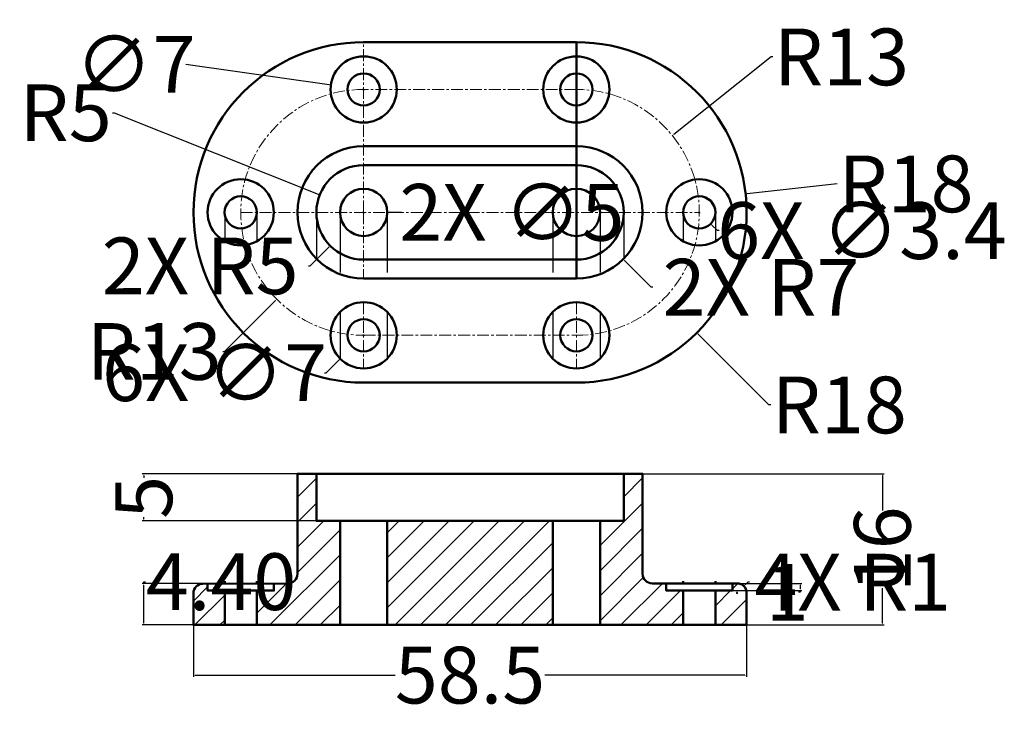
# Model space of a CAD drawing. Units: millimetres. Extents: x 26 to 130, y 11 to 85.
import ezdxf

# ---------------------------------------------------------------- set-up
doc = ezdxf.new("R2010")
doc.units = ezdxf.units.MM
doc.header["$MEASUREMENT"] = 0
doc.linetypes.add('CENTER', pattern=[2, 1.25, -0.25, 0.25, -0.25])
doc.linetypes.add('HIDDEN', pattern=[9.525, 6.35, -3.175])
for name, color, linetype, lineweight in [('M-CNTR', 1, 'CENTER', 18), ('M-DIMS', 2, 'Continuous', 25), ('M-HATC', 8, 'Continuous', 18), ('M-HIDN', 4, 'HIDDEN', 25), ('M-OUTL', 7, 'Continuous', 50)]:
    doc.layers.add(name, color=color, linetype=linetype, lineweight=lineweight)
doc.styles.get("Standard").update_dxf_attribs({"font": 'arial.ttf'})
doc.dimstyles.get("Standard").update_dxf_attribs({"dimtxt": 6, "dimasz": 0.18, "dimexe": 0.18, "dimexo": 0.0625, "dimgap": 0.09, "dimtad": 0, "dimtoh": 1, "dimdec": 0, "dimzin": 0, "dimdsep": 46, "dimtxsty": 'Standard', "dimcen": 0.09, "dimadec": 0, "dimazin": 0, "dimtfac": 1, "dimtdec": 0, "dimtofl": 0, "dimtmove": 0, "dimatfit": 3, "dimfxl": 1, "dimtolj": 1, "dimtzin": 0, "dimarcsym": 0})

# ---------------------------------------------------------------- blocks, each defined once
blk = doc.blocks.new('*D1')
at = {"layer": 'Defpoints', "color": 0, "transparency": 16777216}
for p in [(94.96, 72.32), (84.8, 64.21)]:
    blk.add_point(p, dxfattribs=at)
at = {"layer": 'M-DIMS', "color": 0, "lineweight": -2, "transparency": 16777216}
for p, q in [((105.4, 80.65), (95.1, 72.43)), ((105.58, 80.65), (105.4, 80.65)), ((84.71, 64.21), (84.89, 64.21)), ((84.8, 64.12), (84.8, 64.3))]:
    blk.add_line(p, q, dxfattribs=at)
at = {"layer": 'M-DIMS', "color": 0, "transparency": 16777216}
blk.add_solid([(95.08, 72.45), (95.12, 72.4), (94.96, 72.32)], dxfattribs=at)
at = {"layer": 'M-DIMS', "color": 0, "transparency": 16777216, "insert": (112.84, 80.65), "char_height": 6, "attachment_point": 5}
blk.add_mtext('\\A1;R13', dxfattribs=at)
blk = doc.blocks.new('*D2')
at = {"layer": 'Defpoints', "color": 0, "transparency": 16777216}
for p in [(102.69, 66.16), (84.8, 64.21)]:
    blk.add_point(p, dxfattribs=at)
at = {"layer": 'M-DIMS', "color": 0, "lineweight": -2, "transparency": 16777216}
for p, q in [((112.39, 67.22), (102.87, 66.18)), ((84.71, 64.21), (84.89, 64.21)), ((84.8, 64.12), (84.8, 64.3))]:
    blk.add_line(p, q, dxfattribs=at)
at = {"layer": 'M-DIMS', "color": 0, "transparency": 16777216}
blk.add_solid([(102.87, 66.21), (102.88, 66.15), (102.69, 66.16)], dxfattribs=at)
at = {"layer": 'M-DIMS', "color": 0, "transparency": 16777216, "insert": (119.66, 67.22), "char_height": 6, "attachment_point": 5}
blk.add_mtext('\\A1;R18', dxfattribs=at)
blk = doc.blocks.new('*D3')
at = {"layer": 'Defpoints', "color": 0, "transparency": 16777216}
for p in [(57.66, 66.06), (62.3, 64.21)]:
    blk.add_point(p, dxfattribs=at)
at = {"layer": 'M-DIMS', "color": 0, "lineweight": -2, "transparency": 16777216}
for p, q in [((35.74, 74.74), (35.92, 74.74)), ((35.92, 74.74), (57.49, 66.13)), ((62.21, 64.21), (62.39, 64.21)), ((62.3, 64.12), (62.3, 64.3))]:
    blk.add_line(p, q, dxfattribs=at)
at = {"layer": 'M-DIMS', "color": 0, "transparency": 16777216}
blk.add_solid([(57.5, 66.16), (57.48, 66.1), (57.66, 66.06)], dxfattribs=at)
at = {"layer": 'M-DIMS', "color": 0, "transparency": 16777216, "insert": (30.79, 74.74), "char_height": 6, "attachment_point": 5}
blk.add_mtext('\\A1;R5', dxfattribs=at)
blk = doc.blocks.new('*D4')
at = {"layer": 'Defpoints', "color": 0, "transparency": 16777216}
for p in [(89.8, 36.57), (89.8, 20.57), (117.16, 20.57)]:
    blk.add_point(p, dxfattribs=at)
at = {"layer": 'M-DIMS', "color": 0, "lineweight": -2, "transparency": 16777216}
for p, q in [((89.86, 36.57), (117.34, 36.57)), ((117.16, 36.39), (117.16, 32.68)), ((117.16, 20.75), (117.16, 24.47)), ((89.86, 20.57), (117.34, 20.57))]:
    blk.add_line(p, q, dxfattribs=at)
at = {"layer": 'M-DIMS', "color": 0, "transparency": 16777216}
for points in [[(117.13, 36.39), (117.19, 36.39), (117.16, 36.57)], [(117.13, 20.75), (117.19, 20.75), (117.16, 20.57)]]:
    blk.add_solid(points, dxfattribs=at)
at = {"layer": 'M-DIMS', "color": 0, "transparency": 16777216, "insert": (117.16, 28.57), "char_height": 6, "attachment_point": 5, "rotation": 90}
blk.add_mtext('\\A1;16', dxfattribs=at)
blk = doc.blocks.new('*D5')
at = {"layer": 'Defpoints', "color": 0, "transparency": 16777216}
for p in [(97.3, 24.97), (97.3, 24.21), (108.48, 24.21)]:
    blk.add_point(p, dxfattribs=at)
at = {"layer": 'M-DIMS', "color": 0, "lineweight": -2, "transparency": 16777216}
for p, q in [((97.36, 24.97), (108.66, 24.97)), ((97.36, 24.21), (108.66, 24.21)), ((108.48, 24.03), (108.3, 24.03)), ((108.48, 24.79), (108.48, 24.39)), ((108.48, 24.21), (108.48, 24.03))]:
    blk.add_line(p, q, dxfattribs=at)
at = {"layer": 'M-DIMS', "color": 0, "transparency": 16777216}
for points in [[(108.45, 24.79), (108.51, 24.79), (108.48, 24.97)], [(108.45, 24.39), (108.51, 24.39), (108.48, 24.21)]]:
    blk.add_solid(points, dxfattribs=at)
at = {"layer": 'M-DIMS', "color": 0, "transparency": 16777216, "insert": (107.11, 24.03), "char_height": 6, "attachment_point": 5}
blk.add_mtext('\\A1;1', dxfattribs=at)
blk = doc.blocks.new('*D6')
at = {"layer": 'Defpoints', "color": 0, "transparency": 16777216}
for p in [(58.84, 77.7), (65.77, 76.72)]:
    blk.add_point(p, dxfattribs=at)
at = {"layer": 'M-DIMS', "color": 0, "lineweight": -2, "transparency": 16777216}
for p, q in [((43.48, 79.87), (58.66, 77.72)), ((62.21, 77.21), (62.39, 77.21)), ((62.3, 77.12), (62.3, 77.3))]:
    blk.add_line(p, q, dxfattribs=at)
at = {"layer": 'M-DIMS', "color": 0, "transparency": 16777216}
blk.add_solid([(58.66, 77.75), (58.65, 77.69), (58.84, 77.7)], dxfattribs=at)
at = {"layer": 'M-DIMS', "color": 0, "transparency": 16777216, "insert": (38.16, 79.87), "char_height": 6, "attachment_point": 5}
blk.add_mtext('\\A1;∅7', dxfattribs=at)
blk = doc.blocks.new('HOLE-CBORE-3.4X7')
for radius in [3.5, 1.7]:
    blk.add_circle((62.3, 77.21), radius)
blk = doc.blocks.new('*D8')
at = {"layer": 'Defpoints', "color": 0, "transparency": 16777216}
for p in [(44.3, 20.57), (102.8, 20.57), (102.8, 15.27)]:
    blk.add_point(p, dxfattribs=at)
at = {"layer": 'M-DIMS', "color": 0, "lineweight": -2, "transparency": 16777216}
for p, q in [((44.3, 20.51), (44.3, 15.09)), ((102.8, 20.51), (102.8, 15.09)), ((44.48, 15.27), (65.65, 15.27)), ((102.62, 15.27), (81.46, 15.27))]:
    blk.add_line(p, q, dxfattribs=at)
at = {"layer": 'M-DIMS', "color": 0, "transparency": 16777216}
for points in [[(44.48, 15.3), (44.48, 15.24), (44.3, 15.27)], [(102.62, 15.3), (102.62, 15.24), (102.8, 15.27)]]:
    blk.add_solid(points, dxfattribs=at)
at = {"layer": 'M-DIMS', "color": 0, "transparency": 16777216, "insert": (73.55, 15.27), "char_height": 6, "attachment_point": 5}
blk.add_mtext('\\A1;58.5', dxfattribs=at)
blk = doc.blocks.new('*D9')
at = {"layer": 'Defpoints', "color": 0, "transparency": 16777216}
for p in [(39.05, 24.97), (54.31, 24.97), (44.3, 20.57)]:
    blk.add_point(p, dxfattribs=at)
at = {"layer": 'M-DIMS', "color": 0, "lineweight": -2, "transparency": 16777216}
for p, q in [((39.05, 24.97), (39.05, 25.15)), ((39.05, 25.15), (39.23, 25.15)), ((54.24, 24.97), (38.87, 24.97)), ((39.05, 20.75), (39.05, 24.79)), ((44.24, 20.57), (38.87, 20.57))]:
    blk.add_line(p, q, dxfattribs=at)
at = {"layer": 'M-DIMS', "color": 0, "transparency": 16777216}
for points in [[(39.02, 24.79), (39.08, 24.79), (39.05, 24.97)], [(39.02, 20.75), (39.08, 20.75), (39.05, 20.57)]]:
    blk.add_solid(points, dxfattribs=at)
at = {"layer": 'M-DIMS', "color": 0, "transparency": 16777216, "insert": (47.22, 25.15), "char_height": 6, "attachment_point": 5}
blk.add_mtext('\\A1;4.40', dxfattribs=at)
blk = doc.blocks.new('*D10')
at = {"layer": 'Defpoints', "color": 0, "transparency": 16777216}
for p in [(57.3, 36.57), (39.05, 31.57), (57.3, 31.57)]:
    blk.add_point(p, dxfattribs=at)
at = {"layer": 'M-DIMS', "color": 0, "lineweight": -2, "transparency": 16777216}
for p, q in [((57.24, 36.57), (38.87, 36.57)), ((39.05, 36.39), (39.05, 36.15)), ((57.24, 31.57), (38.87, 31.57)), ((39.05, 31.75), (39.05, 31.99))]:
    blk.add_line(p, q, dxfattribs=at)
at = {"layer": 'M-DIMS', "color": 0, "transparency": 16777216}
for points in [[(39.02, 36.39), (39.08, 36.39), (39.05, 36.57)], [(39.02, 31.75), (39.08, 31.75), (39.05, 31.57)]]:
    blk.add_solid(points, dxfattribs=at)
at = {"layer": 'M-DIMS', "color": 0, "transparency": 16777216, "insert": (39.05, 34.07), "char_height": 6, "attachment_point": 5, "rotation": 90}
blk.add_mtext('\\A1;5', dxfattribs=at)
blk = doc.blocks.new('*D11')
at = {"layer": 'Defpoints', "color": 0, "transparency": 16777216}
for p in [(84.8, 64.21), (97.53, 51.48)]:
    blk.add_point(p, dxfattribs=at)
at = {"layer": 'M-DIMS', "color": 0, "lineweight": -2, "transparency": 16777216}
for p, q in [((84.71, 64.21), (84.89, 64.21)), ((84.8, 64.12), (84.8, 64.3)), ((105.17, 43.84), (97.66, 51.35)), ((105.35, 43.84), (105.17, 43.84))]:
    blk.add_line(p, q, dxfattribs=at)
at = {"layer": 'M-DIMS', "color": 0, "transparency": 16777216}
blk.add_solid([(97.68, 51.37), (97.64, 51.33), (97.53, 51.48)], dxfattribs=at)
at = {"layer": 'M-DIMS', "color": 0, "transparency": 16777216, "insert": (112.61, 43.84), "char_height": 6, "attachment_point": 5}
blk.add_mtext('\\A1;R18', dxfattribs=at)
blk = doc.blocks.new('*D12')
at = {"layer": 'Defpoints', "color": 0, "transparency": 16777216}
for p in [(62.3, 64.21), (53.11, 55.02)]:
    blk.add_point(p, dxfattribs=at)
at = {"layer": 'M-DIMS', "color": 0, "lineweight": -2, "transparency": 16777216}
for p, q in [((62.21, 64.21), (62.39, 64.21)), ((62.3, 64.12), (62.3, 64.3)), ((47.59, 49.5), (52.98, 54.89)), ((47.41, 49.5), (47.59, 49.5))]:
    blk.add_line(p, q, dxfattribs=at)
at = {"layer": 'M-DIMS', "color": 0, "transparency": 16777216}
blk.add_solid([(52.96, 54.91), (53, 54.87), (53.11, 55.02)], dxfattribs=at)
at = {"layer": 'M-DIMS', "color": 0, "transparency": 16777216, "insert": (40.15, 49.5), "char_height": 6, "attachment_point": 5}
blk.add_mtext('\\A1;R13', dxfattribs=at)
blk = doc.blocks.new('*D13')
at = {"layer": 'Defpoints', "color": 0, "transparency": 16777216}
for p in [(84.8, 64.21), (89.75, 59.26)]:
    blk.add_point(p, dxfattribs=at)
at = {"layer": 'M-DIMS', "color": 0, "lineweight": -2, "transparency": 16777216}
for p, q in [((84.71, 64.21), (84.89, 64.21)), ((84.8, 64.12), (84.8, 64.3)), ((92.72, 56.29), (89.88, 59.13)), ((92.9, 56.29), (92.72, 56.29))]:
    blk.add_line(p, q, dxfattribs=at)
at = {"layer": 'M-DIMS', "color": 0, "transparency": 16777216}
blk.add_solid([(89.9, 59.15), (89.86, 59.11), (89.75, 59.26)], dxfattribs=at)
at = {"layer": 'M-DIMS', "color": 0, "transparency": 16777216, "insert": (104.33, 56.29), "char_height": 6, "attachment_point": 5}
blk.add_mtext('\\A1;2X R7', dxfattribs=at)
blk = doc.blocks.new('*D14')
at = {"layer": 'Defpoints', "color": 0, "transparency": 16777216}
for p in [(62.3, 64.21), (58.76, 60.67)]:
    blk.add_point(p, dxfattribs=at)
at = {"layer": 'M-DIMS', "color": 0, "lineweight": -2, "transparency": 16777216}
for p, q in [((62.21, 64.21), (62.39, 64.21)), ((62.3, 64.12), (62.3, 64.3)), ((56.64, 58.55), (58.64, 60.55)), ((56.46, 58.55), (56.64, 58.55))]:
    blk.add_line(p, q, dxfattribs=at)
at = {"layer": 'M-DIMS', "color": 0, "transparency": 16777216}
blk.add_solid([(58.62, 60.57), (58.66, 60.53), (58.76, 60.67)], dxfattribs=at)
at = {"layer": 'M-DIMS', "color": 0, "transparency": 16777216, "insert": (45.01, 58.55), "char_height": 6, "attachment_point": 5}
blk.add_mtext('\\A1;2X R5', dxfattribs=at)
blk = doc.blocks.new('*D15')
at = {"layer": 'Defpoints', "color": 0, "transparency": 16777216}
for p in [(64.78, 53.68), (59.82, 48.73)]:
    blk.add_point(p, dxfattribs=at)
at = {"layer": 'M-DIMS', "color": 0, "lineweight": -2, "transparency": 16777216}
for p, q in [((62.21, 51.21), (62.39, 51.21)), ((62.3, 51.12), (62.3, 51.3)), ((58.34, 47.25), (59.7, 48.61)), ((58.16, 47.25), (58.34, 47.25))]:
    blk.add_line(p, q, dxfattribs=at)
at = {"layer": 'M-DIMS', "color": 0, "transparency": 16777216}
blk.add_solid([(59.68, 48.63), (59.72, 48.59), (59.82, 48.73)], dxfattribs=at)
at = {"layer": 'M-DIMS', "color": 0, "transparency": 16777216, "insert": (46.53, 47.25), "char_height": 6, "attachment_point": 5}
blk.add_mtext('\\A1;6X ∅7', dxfattribs=at)
blk = doc.blocks.new('*D16')
at = {"layer": 'Defpoints', "color": 0, "transparency": 16777216}
for p in [(96.6, 65.41), (99, 63)]:
    blk.add_point(p, dxfattribs=at)
at = {"layer": 'M-DIMS', "color": 0, "lineweight": -2, "transparency": 16777216}
for p, q in [((97.71, 64.21), (97.89, 64.21)), ((97.8, 64.12), (97.8, 64.3)), ((99.72, 62.28), (99.13, 62.87)), ((99.9, 62.28), (99.72, 62.28))]:
    blk.add_line(p, q, dxfattribs=at)
at = {"layer": 'M-DIMS', "color": 0, "transparency": 16777216}
blk.add_solid([(99.15, 62.89), (99.1, 62.85), (99, 63)], dxfattribs=at)
at = {"layer": 'M-DIMS', "color": 0, "transparency": 16777216, "insert": (115, 62.28), "char_height": 6, "attachment_point": 5}
blk.add_mtext('\\A1;6X ∅3.4', dxfattribs=at)
blk = doc.blocks.new('*D17')
at = {"layer": 'Defpoints', "color": 0, "transparency": 16777216}
for p in [(59.8, 64.21), (64.8, 64.21)]:
    blk.add_point(p, dxfattribs=at)
at = {"layer": 'M-DIMS', "color": 0, "lineweight": -2, "transparency": 16777216}
for p, q in [((62.21, 64.21), (62.39, 64.21)), ((62.3, 64.12), (62.3, 64.3)), ((66.3, 64.21), (64.98, 64.21))]:
    blk.add_line(p, q, dxfattribs=at)
at = {"layer": 'M-DIMS', "color": 0, "transparency": 16777216}
blk.add_solid([(64.98, 64.24), (64.98, 64.18), (64.8, 64.21)], dxfattribs=at)
at = {"layer": 'M-DIMS', "color": 0, "transparency": 16777216, "insert": (77.98, 64.21), "char_height": 6, "attachment_point": 5}
blk.add_mtext('\\A1;2X ∅5', dxfattribs=at)
blk = doc.blocks.new('*D18')
at = {"layer": 'Defpoints', "color": 0, "transparency": 16777216}
for p in [(101.8, 23.97), (102.51, 24.68)]:
    blk.add_point(p, dxfattribs=at)
at = {"layer": 'M-DIMS', "color": 0, "lineweight": -2, "transparency": 16777216}
for p, q in [((102.93, 25.1), (102.64, 24.81)), ((103.11, 25.1), (102.93, 25.1)), ((101.71, 23.97), (101.89, 23.97)), ((101.8, 23.88), (101.8, 24.06))]:
    blk.add_line(p, q, dxfattribs=at)
at = {"layer": 'M-DIMS', "color": 0, "transparency": 16777216}
blk.add_solid([(102.61, 24.83), (102.66, 24.79), (102.51, 24.68)], dxfattribs=at)
at = {"layer": 'M-DIMS', "color": 0, "transparency": 16777216, "insert": (114.03, 25.1), "char_height": 6, "attachment_point": 5}
blk.add_mtext('\\A1;4X R1', dxfattribs=at)

msp = doc.modelspace()

# ---------------------------------------------------------------- hatches: boundary and pattern name
at = {"layer": 'M-HATC'}
h = msp.add_hatch(dxfattribs=at)
h.set_pattern_fill('ANSI31', color=256, scale=15)
h.paths.add_polyline_path([(59.801, 31.572), (57.301, 31.572), (57.301, 36.572), (55.301, 36.572), (55.301, 25.968, -0.4128846), (54.306, 24.968), (52.801, 24.961), (52.801, 24.207), (51.001, 24.207), (51.001, 20.572), (59.801, 20.572)])
h.paths.add_polyline_path([(82.301, 31.572), (64.801, 31.572), (64.801, 20.572), (82.301, 20.572)])
h.paths.add_polyline_path([(94.301, 24.972), (92.801, 24.972, -0.4142136), (91.801, 25.972), (91.801, 36.572), (89.801, 36.572), (89.801, 31.572), (87.301, 31.572), (87.301, 20.572), (96.101, 20.572), (96.101, 24.207), (94.301, 24.207)])
h.paths.add_polyline_path([(47.601, 24.207), (45.801, 24.207), (45.801, 24.929), (45.297, 24.927, 0.4128846), (44.301, 23.927), (44.301, 20.572), (47.601, 20.572)])
h.paths.add_polyline_path([(102.801, 23.972, 0.4142136), (101.801, 24.972), (101.301, 24.972), (101.301, 24.207), (99.501, 24.207), (99.501, 20.572), (102.801, 20.572)])

# ---------------------------------------------------------------- linework, layer by layer
at = {"layer": 'M-CNTR'}
for p, q in [((62.301, 64.207), (62.301, 82.207)), ((49.301, 64.207), (97.801, 64.207)), ((62.301, 64.207), (62.301, 57.207)), ((62.301, 54.707), (62.301, 47.707))]:
    msp.add_line(p, q, dxfattribs=at)
msp.add_lwpolyline([(62.301, 51.207), (84.801, 51.207, 1), (84.801, 77.207), (62.301, 77.207, 1)], format="xyb", close=True, dxfattribs=at)
msp.add_lwpolyline([(84.801, 54.707), (84.801, 47.707)], dxfattribs=at)
at = {"layer": 'M-HIDN'}
for p, q in [((47.601, 64.207), (47.601, 61.148)), ((51.001, 64.207), (51.001, 61.148)), ((57.301, 64.207), (57.301, 59.308)), ((59.801, 64.207), (59.801, 57.669)), ((64.801, 64.207), (64.801, 57.207)), ((82.301, 64.207), (82.301, 57.207)), ((87.301, 64.207), (87.301, 57.669)), ((89.801, 64.207), (89.801, 59.308)), ((96.101, 64.207), (96.101, 61.148)), ((99.501, 64.207), (99.501, 61.148)), ((59.801, 53.657), (59.801, 48.758)), ((64.801, 53.657), (64.801, 48.758)), ((82.301, 53.657), (82.301, 48.758)), ((87.301, 53.657), (87.301, 48.758))]:
    msp.add_line(p, q, dxfattribs=at)
at = {"layer": 'M-OUTL'}
for p, q in [((59.801, 31.572), (59.801, 20.572)), ((64.801, 31.572), (64.801, 20.572)), ((82.301, 31.572), (82.301, 20.572)), ((87.301, 31.572), (87.301, 20.572)), ((47.601, 25.207), (47.601, 24.937)), ((51.001, 25.207), (51.001, 24.953)), ((96.101, 25.207), (96.101, 24.972)), ((99.501, 25.207), (99.501, 24.972)), ((47.601, 24.207), (47.601, 20.572)), ((51.001, 24.207), (51.001, 20.572)), ((96.101, 24.207), (96.101, 20.572)), ((99.501, 24.207), (99.501, 20.572))]:
    msp.add_line(p, q, dxfattribs=at)
for points in [[(84.801, 82.207, -1), (84.801, 46.207), (62.301, 46.207, -1), (62.301, 82.207), (84.801, 82.207), (84.801, 64.207), (84.801, 57.207)], [(44.301, 20.572), (102.801, 20.572), (102.801, 23.972, 0.4142136), (101.801, 24.972), (92.801, 24.972, -0.4142136), (91.801, 25.972), (91.801, 36.572), (55.301, 36.572), (55.301, 25.968, -0.4128846), (54.306, 24.968), (45.297, 24.927, 0.4128846), (44.301, 23.927), (44.301, 20.522)]]:
    msp.add_lwpolyline(points, format="xyb", dxfattribs=at)
for points in [[(62.301, 57.207), (84.801, 57.207, 1), (84.801, 71.207), (62.301, 71.207, 1)], [(62.301, 59.207), (84.801, 59.207, 1), (84.801, 69.207), (62.301, 69.207, 1)]]:
    msp.add_lwpolyline(points, format="xyb", close=True, dxfattribs=at)
for points in [[(89.801, 36.572), (89.801, 31.572), (57.301, 31.572), (57.301, 36.572)], [(45.801, 24.929), (45.801, 24.207), (52.801, 24.207), (52.801, 24.961)], [(94.301, 24.972), (94.301, 24.207), (101.301, 24.207), (101.301, 24.972)]]:
    msp.add_lwpolyline(points, dxfattribs=at)
for centre in [(62.301, 64.207), (84.801, 64.207)]:
    msp.add_circle(centre, 2.5, dxfattribs=at)

# ---------------------------------------------------------------- block references
for p in [(0, 0), (22.5, 0), (-13, -13), (35.5, -13), (0, -26)]:
    msp.add_blockref('HOLE-CBORE-3.4X7', p, dxfattribs=at)
at = {"layer": 'M-OUTL', "rotation": 90}
msp.add_blockref('HOLE-CBORE-3.4X7', (162.008, -11.094), dxfattribs=at)

# ---------------------------------------------------------------- dimensions: what is measured, and where the dimension line sits
at = {"layer": 'M-DIMS'}
for center, mpoint, override, picture, middle in [((84.801, 64.207), (94.963, 72.316), {"dimclrd": 0, "dimclre": 0, "dimclrt": 0}, '*D1', (112.843, 80.648)), ((62.301, 64.207), (57.658, 66.061), {"dimclrd": 0, "dimclre": 0, "dimclrt": 0}, '*D3', (30.793, 74.738)), ((84.801, 64.207), (102.695, 66.163), {"dimclrd": 0, "dimclre": 0, "dimclrt": 0}, '*D2', (112.395, 67.224)), ((62.301, 64.207), (53.107, 55.017), {"dimdec": 0, "dimlfac": 1, "dimrnd": 0, "dimzin": 0, "dimdsep": 46, "dimlunit": 2}, '*D12', (40.152, 49.503)), ((84.801, 64.207), (97.53, 51.48), {"dimdec": 0, "dimlfac": 1, "dimrnd": 0, "dimzin": 0, "dimdsep": 46, "dimlunit": 2}, '*D11', (112.612, 43.844))]:
    dim = msp.add_radius_dim(center=center, mpoint=mpoint, dimstyle='Standard', override=override, dxfattribs=at)
    dim.commit()
    dim.dimension.update_dxf_attribs({"geometry": picture, "text_midpoint": middle, "dimtype": 164})
dim = msp.add_diameter_dim_2p(p1=(65.767, 76.717), p2=(58.836, 77.697), dimstyle='Standard', override={"dimclrd": 0, "dimclre": 0, "dimclrt": 0}, dxfattribs=at)
dim.commit()
dim.dimension.update_dxf_attribs({"geometry": '*D6', "text_midpoint": (43.478, 79.87), "dimtype": 163})
for p1, p2, text, override, picture, middle in [((59.801, 64.207), (64.801, 64.207), '2X <>', {"dimdec": 0, "dimlfac": 1, "dimrnd": 0, "dimzin": 0, "dimdsep": 46, "dimlunit": 2}, '*D17', (66.301, 64.207)), ((96.603, 65.413), (98.999, 63.001), '6X <>', {"dimdec": 1, "dimlfac": 1, "dimrnd": 0, "dimzin": 0, "dimdsep": 46, "dimlunit": 2}, '*D16', (115.004, 62.277)), ((64.778, 53.68), (59.824, 48.734), '6X <>', {"dimdec": 0, "dimlfac": 1, "dimrnd": 0, "dimzin": 0, "dimdsep": 46, "dimlunit": 2}, '*D15', (46.535, 47.251))]:
    dim = msp.add_diameter_dim_2p(p1=p1, p2=p2, text=text, dimstyle='Standard', override=override, dxfattribs=at)
    dim.commit()
    dim.dimension.update_dxf_attribs({"geometry": picture, "text_midpoint": middle, "dimtype": 163})
for center, mpoint, text, picture, middle in [((62.301, 64.207), (58.764, 60.674), '2X <>', '*D14', (45.014, 58.554)), ((84.801, 64.207), (89.752, 59.258), '2X <>', '*D13', (104.327, 56.289)), ((101.801, 23.972), (102.508, 24.679), '4X <>', '*D18', (114.028, 25.104))]:
    dim = msp.add_radius_dim(center=center, mpoint=mpoint, text=text, dimstyle='Standard', override={"dimdec": 0, "dimlfac": 1, "dimrnd": 0, "dimzin": 0, "dimdsep": 46, "dimlunit": 2}, dxfattribs=at)
    dim.commit()
    dim.dimension.update_dxf_attribs({"geometry": picture, "text_midpoint": middle, "dimtype": 164})
for base, p1, p2, override, picture, middle in [((39.051, 31.572), (57.301, 36.572), (57.301, 31.572), {"dimdec": 0, "dimlfac": 1, "dimrnd": 0, "dimzin": 0, "dimdsep": 46, "dimlunit": 2}, '*D10', (39.051, 34.072)), ((117.158, 20.572), (89.801, 36.572), (89.801, 20.572), {"dimclrd": 0, "dimclre": 0, "dimclrt": 0}, '*D4', (117.158, 28.572)), ((39.051, 24.968), (44.301, 20.572), (54.306, 24.968), {"dimdec": 2, "dimlfac": 1, "dimrnd": 0, "dimzin": 0, "dimdsep": 46, "dimlunit": 2}, '*D9', (47.224, 25.148)), ((108.482, 24.207), (97.301, 24.972), (97.301, 24.207), {"dimclrd": 0, "dimclre": 0, "dimclrt": 0}, '*D5', (107.107, 24.027))]:
    dim = msp.add_linear_dim(base=base, p1=p1, p2=p2, angle=90, dimstyle='Standard', override=override, dxfattribs=at)
    dim.commit()
    dim.dimension.update_dxf_attribs({"geometry": picture, "text_midpoint": middle})
dim = msp.add_linear_dim(base=(102.801, 15.272), p1=(44.301, 20.572), p2=(102.801, 20.572), dimstyle='Standard', override={"dimdec": 1, "dimlfac": 1, "dimrnd": 0, "dimzin": 0, "dimdsep": 46, "dimlunit": 2}, dxfattribs=at)
dim.commit()
dim.dimension.update_dxf_attribs({"geometry": '*D8', "text_midpoint": (73.551, 15.272)})

doc.saveas('drawing.dxf')
